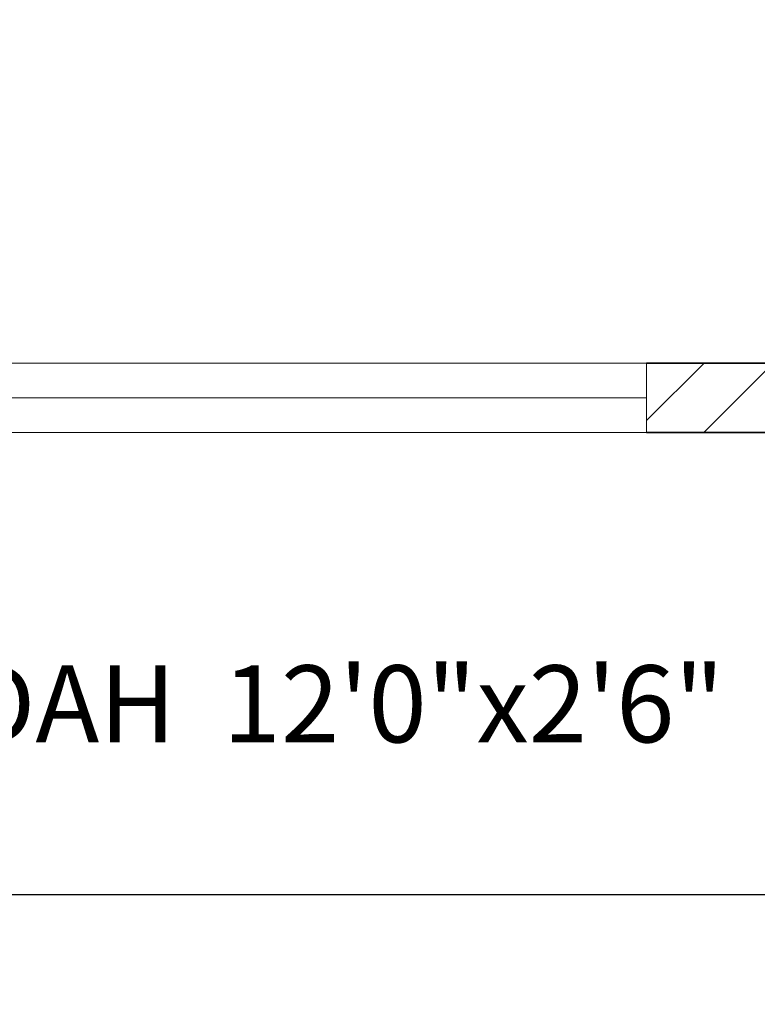
# Model space of a CAD drawing. Units: inches. Extents: x 1885 to 2748, y 783 to 2421.
# Tile 6 of 117: x 2017 to 2065, y 1050 to 1114. Entities that reach past the tile are written whole.
import ezdxf

# ---------------------------------------------------------------- set-up
doc = ezdxf.new("R2010")
doc.units = ezdxf.units.IN
for name, color, linetype, lineweight in [('A-ANNO-DIMS', 2, 'Continuous', 18), ('A-AREA-IDEN', 7, 'Continuous', 18), ('A-FLOR-BALC', 7, 'Continuous', 25), ('A-GLAZ', 181, 'Continuous', 18), ('A-WALL', 7, 'Continuous', 35)]:
    doc.layers.add(name, color=color, linetype=linetype, lineweight=lineweight)
doc.layers.add('A-WALL-PATT', color=85, linetype='Continuous', lineweight=13, true_color=0x58ba48)
doc.styles.get("Standard").update_dxf_attribs({"font": 'arial.ttf'})
doc.dimstyles.get("Standard").update_dxf_attribs({"dimtxt": 0.18, "dimasz": 0.18, "dimexe": 0.18, "dimexo": 0.0625, "dimgap": 0.09, "dimtad": 0, "dimtih": 1, "dimtoh": 1, "dimdec": 4, "dimzin": 0, "dimdsep": 46, "dimtxsty": 'Standard', "dimcen": 0.09, "dimadec": 0, "dimazin": 0, "dimtfac": 1, "dimtdec": 4, "dimtofl": 0, "dimtmove": 0, "dimatfit": 3, "dimfxl": 1, "dimtolj": 1, "dimtzin": 0, "dimarcsym": 0})

# ---------------------------------------------------------------- blocks, each defined once
blk = doc.blocks.new('WIN-60')
for p, q in [((0.004, 59.998), (4.504, 59.998)), ((0.004, 59.998), (0.004, -0.002)), ((4.504, 59.998), (2.254, 59.998)), ((2.254, 59.998), (2.254, -0.002)), ((4.504, -0.002), (4.504, 59.998)), ((2.254, -0.002), (0.004, -0.002)), ((0.004, -0.002), (4.504, -0.002))]:
    blk.add_line(p, q)
blk = doc.blocks.new('*D43')
at = {"layer": 'A-ANNO-DIMS', "color": 0, "lineweight": -2, "transparency": 16777216}
for p, q in [((1971.274, 1057.443), (1971.274, 922.479)), ((2618.274, 1057.443), (2618.274, 922.479)), ((1971.454, 922.659), (2294.484, 922.659)), ((2618.094, 922.659), (2295.063, 922.659))]:
    blk.add_line(p, q, dxfattribs=at)
at = {"layer": 'A-ANNO-DIMS', "color": 0, "transparency": 16777216}
for points in [[(1971.454, 922.689), (1971.454, 922.629), (1971.274, 922.659)], [(2618.094, 922.689), (2618.094, 922.629), (2618.274, 922.659)]]:
    blk.add_solid(points, dxfattribs=at)
at = {"layer": 'Defpoints', "color": 0, "transparency": 16777216}
for p in [(1971.274, 1057.506), (2618.274, 1057.506), (2618.274, 922.659)]:
    blk.add_point(p, dxfattribs=at)
at = {"layer": 'A-ANNO-DIMS', "color": 0, "transparency": 16777216, "insert": (2294.774, 922.659), "char_height": 0.18, "attachment_point": 5}
blk.add_mtext('\\A1;647', dxfattribs=at)

msp = doc.modelspace()

# ---------------------------------------------------------------- hatches: boundary and pattern name
at = {"layer": 'A-WALL-PATT'}
h = msp.add_hatch(dxfattribs=at)
h.set_pattern_fill('ANSI32', color=256)
h.paths.add_polyline_path([(2007.772, 2318.006), (1980.774, 2318.006), (1980.774, 2281.215), (1985.274, 2281.215), (1985.274, 2313.506), (2007.772, 2313.506), (2007.772, 2315.756)])
h.paths.add_polyline_path([(2094.324, 2318.006), (2067.772, 2318.006), (2067.772, 2313.506), (2094.324, 2313.506), (2094.324, 2315.756)])
h.paths.add_polyline_path([(2131.367, 2315.756), (2131.367, 2318.006), (2131.189, 2318.006), (2112.609, 2318.006), (2112.609, 2313.506), (2117.274, 2313.506), (2117.274, 2255.201), (2121.774, 2255.201), (2121.774, 2313.506), (2131.367, 2313.506)])
h.paths.add_polyline_path([(2190.512, 2318.006), (2155.367, 2318.006), (2155.367, 2313.506), (2169.774, 2313.506), (2169.774, 2229.506), (2121.774, 2229.506), (2121.774, 2233.451), (2119.524, 2233.451), (2117.274, 2233.451), (2117.274, 2201.101), (2121.774, 2201.101), (2121.774, 2225.006), (2169.774, 2225.006), (2169.774, 2165.006), (2306.274, 2165.006), (2306.274, 2066.006), (2310.774, 2066.006), (2344.274, 2066.006), (2486.274, 2066.006), (2486.274, 1886.006), (2483.02, 1886.006), (2483.02, 1881.506), (2486.274, 1881.506), (2486.274, 1880.678), (2490.774, 1880.678), (2490.774, 2070.506), (2344.274, 2070.506), (2310.774, 2070.506), (2310.774, 2165.006), (2310.774, 2173.636), (2308.524, 2173.636), (2306.274, 2173.636), (2306.274, 2169.506), (2174.274, 2169.506), (2174.274, 2313.506), (2190.512, 2313.506), (2190.512, 2315.756)])
h.paths.add_polyline_path([(1985.274, 2221.215), (1980.774, 2221.215), (1980.774, 2165.006), (1992.774, 2165.006), (1992.774, 2141.927), (1997.274, 2141.927), (1997.274, 2165.006), (2117.274, 2165.006), (2117.274, 2163.126), (2121.774, 2163.126), (2121.774, 2172.734), (2119.524, 2172.734), (2117.274, 2172.734), (2117.274, 2169.506), (1985.274, 2169.506)])
h.paths.add_polyline_path([(1997.274, 2105.927), (1992.774, 2105.927), (1992.774, 2070.506), (2016.774, 2070.506), (2016.774, 2059.123), (2019.024, 2059.123), (2021.274, 2059.123), (2021.274, 2070.506), (2117.274, 2070.506), (2117.274, 2022.506), (2114.423, 2022.506), (2114.423, 2018.006), (2123.627, 2018.006), (2123.627, 2020.256), (2123.627, 2022.506), (2121.774, 2022.506), (2121.774, 2142.587), (2119.524, 2142.587), (2117.274, 2142.587), (2117.274, 2075.006), (1997.274, 2075.006)])
h.paths.add_polyline_path([(2092.029, 2020.256), (2092.029, 2022.506), (2021.274, 2022.506), (2021.274, 2035.123), (2016.774, 2035.123), (2016.774, 2018.006), (2016.774, 1978.784), (2021.274, 1978.784), (2021.274, 2018.006), (2092.029, 2018.006)])
h.paths.add_polyline_path([(2260.938, 2022.506), (2153.105, 2022.506), (2153.105, 2020.256), (2153.105, 2018.006), (2155.274, 2018.006), (2155.274, 1886.006), (2107.629, 1886.006), (2107.629, 1881.506), (2182.911, 1881.506), (2182.911, 1883.756), (2182.911, 1886.006), (2159.774, 1886.006), (2159.774, 2018.006), (2260.938, 2018.006), (2260.938, 2020.256)])
h.paths.add_polyline_path([(2047.629, 1883.756), (2047.629, 1886.006), (2021.274, 1886.006), (2021.274, 1918.784), (2019.024, 1918.784), (2016.774, 1918.784), (2016.774, 1881.506), (2047.629, 1881.506)])
h.paths.add_polyline_path([(2306.361, 1883.756), (2306.361, 1886.006), (2296.274, 1886.006), (2296.274, 1982.006), (2316.535, 1982.006), (2316.535, 1984.256), (2316.535, 1986.506), (2296.274, 1986.506), (2296.274, 2022.506), (2289.276, 2022.506), (2289.276, 2018.006), (2291.774, 2018.006), (2291.774, 1886.006), (2242.911, 1886.006), (2242.911, 1881.506), (2306.361, 1881.506)], flags=17)
h.paths.add_polyline_path([(1985.274, 1843.006), (2021.6, 1843.006), (2021.534, 1845.441), (2021.477, 1847.506), (1980.774, 1847.506), (1980.774, 1809.446), (1985.274, 1809.446)])
h.paths.add_polyline_path([(2131.482, 1845.256), (2131.482, 1847.506), (2081.534, 1847.506), (2081.534, 1843.006), (2117.274, 1843.006), (2117.274, 1784.147), (2119.524, 1784.147), (2121.774, 1784.147), (2121.774, 1843.006), (2131.482, 1843.006)])
h.paths.add_polyline_path([(2203.886, 1847.506), (2155.482, 1847.506), (2155.482, 1843.006), (2169.774, 1843.006), (2169.774, 1759.006), (2121.774, 1759.006), (2121.774, 1761.457), (2117.274, 1761.457), (2117.274, 1730.429), (2121.774, 1730.429), (2121.774, 1754.506), (2177.421, 1754.506), (2177.421, 1756.756), (2177.421, 1759.006), (2174.274, 1759.006), (2174.274, 1843.006), (2203.886, 1843.006)])
h.paths.add_polyline_path([(2335.554, 1845.256), (2335.554, 1847.506), (2239.886, 1847.506), (2239.886, 1843.006), (2306.274, 1843.006), (2306.274, 1759.006), (2199.486, 1759.006), (2199.486, 1754.506), (2310.774, 1754.506), (2310.774, 1843.006), (2335.554, 1843.006)])
h.paths.add_polyline_path([(2348.774, 2022.506), (2344.274, 2022.506), (2344.274, 1986.506), (2341.681, 1986.506), (2341.681, 1982.006), (2344.274, 1982.006), (2344.274, 1886.006), (2330.361, 1886.006), (2330.361, 1881.506), (2361.627, 1881.506), (2361.627, 1883.756), (2361.627, 1886.006), (2348.774, 1886.006)], flags=17)
h.paths.add_polyline_path([(2283.251, 2315.756), (2283.251, 2318.006), (2238.512, 2318.006), (2238.512, 2313.506), (2283.251, 2313.506)], flags=17)
h.paths.add_polyline_path([(2363.274, 2348.006), (2388.677, 2348.006), (2388.677, 2350.256), (2388.677, 2352.506), (2358.774, 2352.506), (2358.774, 2348.006), (2358.774, 2318.006), (2344.481, 2318.006), (2344.481, 2313.506), (2358.774, 2313.506), (2358.774, 2229.506), (2310.774, 2229.506), (2310.774, 2231.952), (2306.274, 2231.952), (2306.274, 2205.611), (2310.774, 2205.611), (2310.774, 2225.006), (2358.774, 2225.006), (2358.774, 2211.506), (2452.329, 2211.506), (2452.329, 2213.756), (2452.329, 2216.006), (2363.274, 2216.006), (2363.274, 2318.006)])
h.paths.add_polyline_path([(2310.774, 2313.506), (2320.481, 2313.506), (2320.481, 2315.756), (2320.481, 2318.006), (2302.728, 2318.006), (2302.728, 2313.506), (2306.274, 2313.506), (2306.274, 2251.076), (2310.774, 2251.076)], flags=17)
h.paths.add_polyline_path([(2490.774, 2352.506), (2486.274, 2352.506), (2448.677, 2352.506), (2448.677, 2348.006), (2486.274, 2348.006), (2486.274, 2318.006), (2486.274, 2216.006), (2481.78, 2216.006), (2481.78, 2211.506), (2486.274, 2211.506), (2486.274, 2165.006), (2493.289, 2165.006), (2493.289, 2167.256), (2493.289, 2169.506), (2490.774, 2169.506), (2490.774, 2313.506), (2494.429, 2313.506), (2494.429, 2318.006), (2490.774, 2318.006)])
h.paths.add_polyline_path([(2534.653, 2318.006), (2515.691, 2318.006), (2515.691, 2313.506), (2534.653, 2313.506), (2534.653, 2315.756)])
h.paths.add_polyline_path([(2618.274, 2318.006), (2594.653, 2318.006), (2594.653, 2313.506), (2613.774, 2313.506), (2613.774, 2281.706), (2618.274, 2281.706)])
h.paths.add_polyline_path([(2618.274, 2221.706), (2613.774, 2221.706), (2613.774, 2169.506), (2554.019, 2169.506), (2554.019, 2165.006), (2613.774, 2165.006), (2613.774, 2152.878), (2618.274, 2152.878)])
h.paths.add_polyline_path([(2618.274, 2128.878), (2616.024, 2128.878), (2613.774, 2128.878), (2613.774, 2117.006), (2529.774, 2117.006), (2529.774, 2165.006), (2532.848, 2165.006), (2532.848, 2169.506), (2522.867, 2169.506), (2522.867, 2165.006), (2525.274, 2165.006), (2525.274, 2117.006), (2525.274, 2112.506), (2525.274, 2108.576), (2529.774, 2108.576), (2529.774, 2112.506), (2613.774, 2112.506), (2613.774, 2080.19), (2618.274, 2080.19)])
h.paths.add_polyline_path([(2618.274, 2044.19), (2616.024, 2044.19), (2613.774, 2044.19), (2613.774, 2015.506), (2529.774, 2015.506), (2529.774, 2088.582), (2527.524, 2088.582), (2525.274, 2088.582), (2525.274, 2011.006), (2613.774, 2011.006), (2613.774, 1956.755), (2618.274, 1956.755)])
h.paths.add_polyline_path([(2618.274, 1881.506), (2618.274, 1896.755), (2613.774, 1896.755), (2613.774, 1881.506), (2613.774, 1847.506), (2592.715, 1847.506), (2592.715, 1843.006), (2613.774, 1843.006), (2613.774, 1765.006), (2613.774, 1760.506), (2609.621, 1760.506), (2609.621, 1756.006), (2613.774, 1756.006), (2613.774, 1660.006), (2608.544, 1660.006), (2608.544, 1655.506), (2613.774, 1655.506), (2613.774, 1508.158), (2618.274, 1508.158)])
h.paths.add_polyline_path([(2565.774, 1843.006), (2568.997, 1843.006), (2568.997, 1847.506), (2490.774, 1847.506), (2490.774, 1849.7), (2488.524, 1849.7), (2486.274, 1849.7), (2486.274, 1847.506), (2477.274, 1847.506), (2477.274, 1838.506), (2477.274, 1821.493), (2486.274, 1821.493), (2486.274, 1838.506), (2561.274, 1838.506), (2561.274, 1765.006), (2486.274, 1765.006), (2486.274, 1786.157), (2477.274, 1786.157), (2477.274, 1765.006), (2477.274, 1756.006), (2486.274, 1756.006), (2565.774, 1756.006), (2585.621, 1756.006), (2585.621, 1758.256), (2585.621, 1760.506), (2565.774, 1760.506), (2565.774, 1765.006)])
h.paths.add_polyline_path([(2486.274, 1651.006), (2561.274, 1651.006), (2561.274, 1567.006), (2486.274, 1567.006), (2486.274, 1591.321), (2477.274, 1591.321), (2477.274, 1567.006), (2477.274, 1558.006), (2477.274, 1555.439), (2481.774, 1555.439), (2481.774, 1558.006), (2568.653, 1558.006), (2568.653, 1560.256), (2568.653, 1562.506), (2565.774, 1562.506), (2565.774, 1655.506), (2584.544, 1655.506), (2584.544, 1657.756), (2584.544, 1660.006), (2565.774, 1660.006), (2486.274, 1660.006), (2477.274, 1660.006), (2477.274, 1651.006), (2477.274, 1632.989), (2486.274, 1632.989)])
h.paths.add_polyline_path([(2449.967, 1883.756), (2449.967, 1886.006), (2421.627, 1886.006), (2421.627, 1881.506), (2449.967, 1881.506)], flags=17)
h.paths.add_polyline_path([(2447.274, 1847.506), (2395.554, 1847.506), (2395.554, 1843.006), (2442.774, 1843.006), (2442.774, 1809.27), (2447.274, 1809.27)])
h.paths.add_polyline_path([(1985.274, 1749.446), (1980.774, 1749.446), (1980.774, 1694.504), (1985.274, 1694.504), (1985.274, 1694.506), (1986.897, 1694.506), (1986.897, 1697.78), (1986.897, 1699.006), (1985.274, 1699.006)])
h.paths.add_polyline_path([(2152.774, 1699.006), (2121.774, 1699.006), (2121.774, 1703.668), (2119.524, 1703.668), (2117.274, 1703.668), (2117.274, 1699.006), (2009.219, 1699.006), (2009.219, 1694.506), (2148.274, 1694.506), (2148.274, 1692.631), (2152.774, 1692.631)])
h.paths.add_polyline_path([(2016.274, 1694.506), (2011.774, 1694.506), (2011.774, 1558.006), (2040.806, 1558.006), (2040.806, 1560.256), (2040.806, 1562.506), (2016.274, 1562.506)])
h.paths.add_polyline_path([(2152.774, 1663.017), (2150.524, 1663.017), (2148.274, 1663.017), (2148.274, 1562.506), (2100.806, 1562.506), (2100.806, 1558.006), (2165.119, 1558.006), (2165.119, 1560.256), (2165.119, 1562.506), (2152.774, 1562.506), (2152.774, 1610.506), (2224.774, 1610.506), (2224.774, 1607.99), (2229.274, 1607.99), (2229.274, 1615.006), (2152.774, 1615.006)])
h.paths.add_polyline_path([(2238.613, 1560.256), (2238.613, 1562.506), (2229.274, 1562.506), (2229.274, 1588.756), (2227.024, 1588.763), (2224.774, 1588.771), (2224.774, 1562.506), (2189.119, 1562.506), (2189.119, 1558.006), (2238.613, 1558.006)])
h.paths.add_polyline_path([(2336.024, 1560.256), (2336.024, 1562.506), (2310.774, 1562.506), (2310.774, 1656.347), (2308.524, 1656.347), (2306.274, 1656.347), (2306.274, 1562.506), (2286.613, 1562.506), (2286.613, 1558.006), (2336.024, 1558.006)])
h.paths.add_polyline_path([(2447.274, 1690.968), (2445.024, 1690.968), (2442.774, 1690.968), (2442.774, 1687.006), (2306.274, 1687.006), (2306.274, 1680.75), (2310.774, 1680.75), (2310.774, 1682.506), (2442.774, 1682.506), (2442.774, 1562.506), (2396.024, 1562.506), (2396.024, 1558.006), (2447.274, 1558.006)])
h.paths.add_polyline_path([(2447.274, 1749.27), (2445.024, 1749.27), (2442.774, 1749.27), (2442.774, 1717.232), (2447.274, 1717.232)])
h.paths.add_polyline_path([(2044.674, 1521.756), (2044.674, 1524.006), (2007.274, 1524.006), (2007.274, 1503.49), (2009.524, 1503.49), (2011.774, 1503.49), (2011.774, 1519.506), (2044.674, 1519.506)])
h.paths.add_polyline_path([(2177.969, 1521.756), (2177.969, 1524.006), (2104.674, 1524.006), (2104.674, 1519.506), (2145.774, 1519.506), (2145.774, 1387.506), (2143.37, 1387.506), (2143.37, 1383.006), (2251.585, 1383.006), (2251.585, 1385.256), (2251.585, 1387.506), (2150.274, 1387.506), (2150.274, 1519.506), (2177.969, 1519.506)])
h.paths.add_polyline_path([(2298.704, 1524.006), (2237.969, 1524.006), (2237.969, 1519.506), (2282.274, 1519.506), (2282.274, 1387.506), (2279.683, 1387.506), (2279.683, 1383.006), (2286.774, 1383.006), (2286.774, 1419.006), (2312.451, 1419.006), (2312.451, 1421.256), (2312.451, 1423.506), (2286.774, 1423.506), (2286.774, 1519.506), (2298.704, 1519.506), (2298.704, 1521.722)], flags=17)
h.paths.add_polyline_path([(2361.897, 1521.756), (2361.897, 1524.006), (2322.704, 1524.006), (2322.704, 1519.506), (2334.774, 1519.506), (2334.774, 1423.506), (2331.93, 1423.506), (2331.93, 1419.006), (2334.774, 1419.006), (2334.774, 1387.506), (2334.774, 1383.228), (2339.274, 1383.228), (2339.274, 1387.506), (2339.274, 1519.506), (2361.897, 1519.506)], flags=17)
h.paths.add_polyline_path([(2447.274, 1521.756), (2447.274, 1524.006), (2421.897, 1524.006), (2421.897, 1519.506), (2447.274, 1519.506)], flags=17)
h.paths.add_polyline_path([(2481.774, 1529.6), (2479.524, 1529.6), (2477.274, 1529.6), (2477.274, 1524.006), (2474.489, 1524.006), (2474.489, 1519.506), (2477.274, 1519.506), (2477.274, 1334.506), (2296.774, 1334.506), (2296.774, 1240.506), (2160.274, 1240.506), (2160.274, 1180.506), (2112.274, 1180.506), (2112.274, 1207.692), (2110.024, 1207.692), (2107.774, 1207.692), (2107.774, 1171.609), (2112.274, 1171.609), (2112.274, 1176.006), (2160.274, 1176.006), (2160.274, 1092.006), (2144.221, 1092.006), (2144.221, 1087.506), (2189.497, 1087.506), (2189.497, 1089.756), (2189.497, 1092.006), (2164.774, 1092.006), (2164.774, 1236.006), (2296.774, 1236.006), (2296.774, 1231.912), (2301.274, 1231.912), (2301.274, 1330.006), (2481.774, 1330.006), (2481.774, 1387.506)])
h.paths.add_polyline_path([(2618.274, 1448.158), (2613.774, 1448.158), (2613.774, 1382.506), (2529.774, 1382.506), (2525.274, 1382.506), (2525.274, 1307.062), (2529.774, 1307.062), (2529.774, 1378.006), (2613.774, 1378.006), (2613.774, 1354.988), (2618.274, 1354.988)])
h.paths.add_polyline_path([(2618.274, 1318.988), (2613.774, 1318.988), (2613.774, 1281.006), (2529.774, 1281.006), (2529.774, 1283.786), (2527.524, 1283.786), (2525.274, 1283.786), (2525.274, 1228.506), (2516.794, 1228.506), (2516.794, 1224.006), (2533.484, 1224.006), (2533.484, 1226.256), (2533.484, 1228.506), (2529.774, 1228.506), (2529.774, 1276.506), (2613.774, 1276.506), (2613.774, 1266.02), (2618.274, 1266.02)])
h.paths.add_polyline_path([(2618.274, 1134.964), (2613.774, 1134.964), (2613.774, 1092.006), (2594.545, 1092.006), (2594.545, 1087.506), (2618.274, 1087.506)])
h.paths.add_polyline_path([(2534.545, 1092.006), (2509.765, 1092.006), (2509.765, 1087.506), (2534.545, 1087.506), (2534.545, 1089.756)])
h.paths.add_polyline_path([(2481.274, 1224.006), (2484.117, 1224.006), (2484.117, 1226.256), (2484.117, 1228.506), (2476.774, 1228.506), (2476.774, 1198.506), (2471.61, 1198.506), (2471.61, 1194.006), (2476.774, 1194.006), (2476.774, 1062.006), (2436.894, 1062.006), (2436.894, 1057.506), (2476.774, 1057.506), (2481.274, 1057.506), (2481.274, 1062.006), (2481.274, 1087.506), (2485.354, 1087.506), (2485.354, 1089.756), (2485.354, 1092.006), (2481.274, 1092.006), (2481.274, 1117.506)])
h.paths.add_polyline_path([(2439.898, 1198.506), (2349.274, 1198.506), (2349.274, 1194.006), (2349.274, 1180.506), (2301.274, 1180.506), (2301.274, 1201.896), (2299.024, 1201.896), (2296.774, 1201.896), (2296.774, 1172.335), (2299.024, 1172.335), (2301.274, 1172.335), (2301.274, 1176.006), (2349.274, 1176.006), (2349.274, 1092.006), (2334.452, 1092.006), (2334.452, 1087.506), (2349.274, 1087.506), (2349.274, 1057.506), (2353.774, 1057.506), (2376.894, 1057.506), (2376.894, 1059.756), (2376.894, 1062.006), (2353.774, 1062.006), (2353.774, 1087.506), (2353.774, 1180.506), (2353.774, 1194.006), (2439.898, 1194.006), (2439.898, 1196.256)])
h.paths.add_polyline_path([(2270.596, 1089.756), (2270.596, 1092.006), (2249.497, 1092.006), (2249.497, 1087.506), (2270.596, 1087.506)], flags=17)
h.paths.add_polyline_path([(2310.452, 1092.006), (2301.274, 1092.006), (2301.274, 1153.292), (2296.774, 1153.292), (2296.774, 1092.006), (2293.786, 1092.006), (2293.786, 1087.506), (2310.452, 1087.506), (2310.452, 1089.756)], flags=17)
h.paths.add_polyline_path([(2112.274, 1150.328), (2110.024, 1150.328), (2107.774, 1150.328), (2107.774, 1092.006), (2104.465, 1092.006), (2104.465, 1087.506), (2120.221, 1087.506), (2120.221, 1089.756), (2120.221, 1092.006), (2112.274, 1092.006)])
h.paths.add_polyline_path([(2082.172, 1092.006), (2058.144, 1092.006), (2058.144, 1087.506), (2082.172, 1087.506), (2082.172, 1089.756)])
h.paths.add_polyline_path([(1975.774, 1145.638), (1971.274, 1145.638), (1971.274, 1087.506), (1980.774, 1087.506), (1998.144, 1087.506), (1998.144, 1089.756), (1998.144, 1092.006), (1985.274, 1092.006), (1975.774, 1092.006)])
h.paths.add_polyline_path([(2112.274, 1244.385), (2110.024, 1244.385), (2107.774, 1244.385), (2107.774, 1240.506), (1992.274, 1240.506), (1992.274, 1271.008), (1987.774, 1271.008), (1987.774, 1240.506), (1980.774, 1240.506), (1975.774, 1240.506), (1971.274, 1240.506), (1971.274, 1205.638), (1975.774, 1205.638), (1975.774, 1236.006), (2107.774, 1236.006), (2107.774, 1233.444), (2112.274, 1233.444), (2112.274, 1236.006)])
h.paths.add_polyline_path([(2112.274, 1383.006), (2114.783, 1383.006), (2114.783, 1385.256), (2114.783, 1387.506), (2102.476, 1387.506), (2102.476, 1383.006), (2107.774, 1383.006), (2107.774, 1335.006), (2011.774, 1335.006), (2011.774, 1349.939), (2007.274, 1349.939), (2007.274, 1335.006), (1987.774, 1335.006), (1987.774, 1330.506), (1987.774, 1307.008), (1992.274, 1307.008), (1992.274, 1330.506), (2007.274, 1330.506), (2107.774, 1330.506), (2107.774, 1264.711), (2112.274, 1264.711)])
h.paths.add_polyline_path([(2077.857, 1387.506), (2011.774, 1387.506), (2011.774, 1390.036), (2009.524, 1390.036), (2007.274, 1390.036), (2007.274, 1373.939), (2011.774, 1373.939), (2011.774, 1383.006), (2077.857, 1383.006)])
h.paths.add_polyline_path([(2011.774, 1443.49), (2007.274, 1443.49), (2007.274, 1410.248), (2011.774, 1410.248)])

# ---------------------------------------------------------------- linework, layer by layer
at = {"layer": 'A-FLOR-BALC'}
msp.add_line((1971.274, 1057.506), (2112.274, 1057.506), dxfattribs=at)
at = {"layer": 'A-WALL'}
for p, q in [((2082.172, 1092.006), (2058.144, 1092.006)), ((2083.698, 1087.506), (2058.144, 1087.506))]:
    msp.add_line(p, q, dxfattribs=at)

# ---------------------------------------------------------------- block references
at = {"layer": 'A-GLAZ', "extrusion": (0, 0, -1), "zscale": -1, "rotation": 90}
msp.add_blockref('WIN-60', (-1998.146, 1087.502), dxfattribs=at)

# ---------------------------------------------------------------- texts
at = {"layer": 'A-AREA-IDEN', "insert": (1992.384, 1072.38), "char_height": 5, "attachment_point": 1}
msp.add_mtext_dynamic_manual_height_columns('VERANDAH  12\'0"x2\'6"', width=123.4564, gutter_width=12.5, heights=[0], dxfattribs=at)

# ---------------------------------------------------------------- dimensions: what is measured, and where the dimension line sits
at = {"layer": 'A-ANNO-DIMS'}
dim = msp.add_linear_dim(base=(2618.274, 922.659), p1=(1971.274, 1057.506), p2=(2618.274, 1057.506), dimstyle='Standard', override={"dimdec": 0, "dimlfac": 1, "dimrnd": 0, "dimzin": 0, "dimdsep": 46, "dimlunit": 2}, dxfattribs=at)
dim.commit()
dim.dimension.update_dxf_attribs({"geometry": '*D43', "text_midpoint": (2294.774, 922.659)})

doc.saveas('drawing.dxf')
